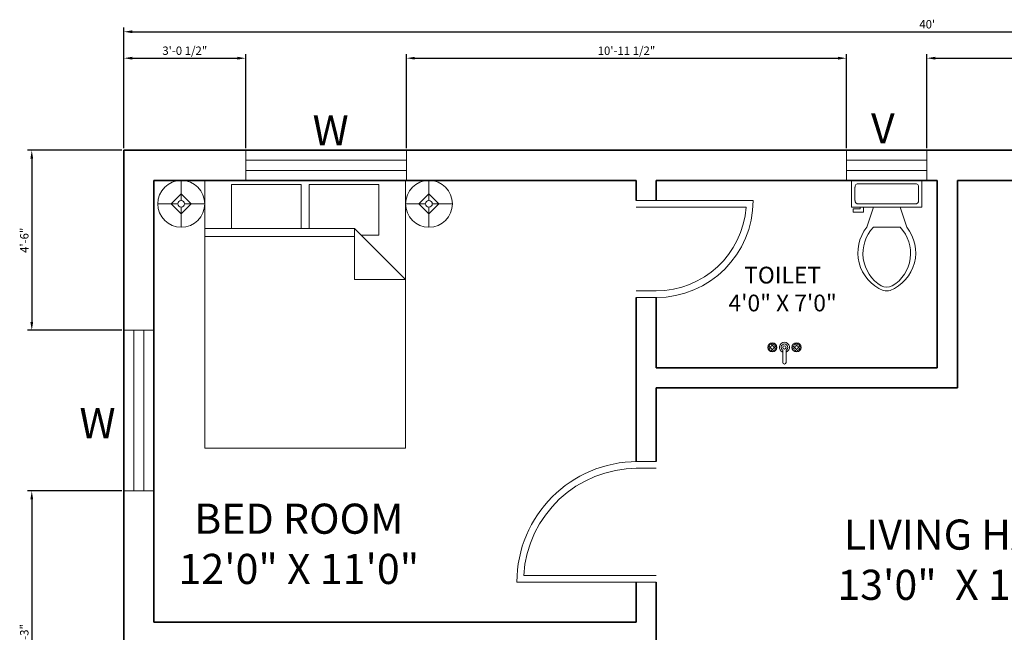
# Model space of a CAD drawing. Units: inches. Extents: x 1025 to 3479, y 1594 to 2212.
# Tile 8 of 9: x 2932 to 3226, y 1957 to 2140. Entities that reach past the tile are written whole.
import ezdxf

# ---------------------------------------------------------------- set-up
doc = ezdxf.new("R2010")
doc.units = ezdxf.units.IN
for name, color, linetype, lineweight in [('A-ANNO-DIMS', 1, 'Continuous', 18), ('A-ANNO-TEXT', 7, 'Continuous', 18), ('A-AREA-IDEN', 4, 'Continuous', 18), ('A-DOOR', 4, 'Continuous', 18), ('A-FLOR-FIXT', 9, 'Continuous', 18), ('A-FURN', 8, 'Continuous', 13), ('A-GLAZ', 3, 'Continuous', 18), ('A-WALL', 7, 'Continuous', 35)]:
    doc.layers.add(name, color=color, linetype=linetype, lineweight=lineweight)
doc.styles.get("Standard").update_dxf_attribs({"font": 'arial.ttf'})
doc.dimstyles.new('ISO-25', dxfattribs={"dimtxt": 2.5, "dimasz": 2.5, "dimexe": 1.25, "dimexo": 0.625, "dimtad": 1, "dimdec": 0, "dimlunit": 3, "dimtxsty": 'Standard', "dimcen": 2.5, "dimadec": 0, "dimazin": 0, "dimtfac": 1, "dimtdec": 0, "dimtmove": 0, "dimatfit": 3, "dimfxl": 1, "dimarcsym": 0})

# ---------------------------------------------------------------- blocks, each defined once
blk = doc.blocks.new('*D3')
at = {"layer": 'A-ANNO-DIMS', "color": 0, "lineweight": -2, "transparency": 16777216}
for p, q in [((2962.75, 2102.12), (2962.75, 2138.14)), ((2965.25, 2136.89), (3440.25, 2136.89)), ((3442.75, 2102.12), (3442.75, 2138.14))]:
    blk.add_line(p, q, dxfattribs=at)
at = {"layer": 'A-ANNO-DIMS', "color": 0, "transparency": 16777216}
for points in [[(2965.25, 2137.31), (2965.25, 2136.48), (2962.75, 2136.89)], [(3440.25, 2137.31), (3440.25, 2136.48), (3442.75, 2136.89)]]:
    blk.add_solid(points, dxfattribs=at)
at = {"layer": 'Defpoints', "color": 0, "transparency": 16777216}
for p in [(3442.75, 2136.89), (2962.75, 2101.49), (3442.75, 2101.49)]:
    blk.add_point(p, dxfattribs=at)
at = {"layer": 'A-ANNO-DIMS', "color": 0, "transparency": 16777216, "insert": (3202.75, 2138.8), "char_height": 2.5, "attachment_point": 5}
blk.add_mtext("40'", dxfattribs=at)
blk = doc.blocks.new('Bed - Queen')
for p, q in [((0, -80.00003), (0, 0)), ((0, 0), (59.99999, 0)), ((59.99999, 0), (59.99999, -80.00003)), ((7.99999, -1.2), (28.79998, -1.2)), ((7.99999, -14.4), (7.99999, -1.2)), ((28.79998, -1.2), (28.79998, -14.4)), ((31.19999, -1.2), (51.99999, -1.2)), ((31.19999, -14.4), (31.19999, -1.2)), ((51.99999, -1.2), (51.99999, -16.4)), ((0, -14.4), (44.8, -14.4)), ((59.99999, -29.6), (44.8, -14.4)), ((44.8, -14.4), (44.8, -29.6)), ((44.8, -16.8), (0, -16.8)), ((51.99999, -16.4), (46.79936, -16.4)), ((44.8, -29.6), (59.99999, -29.6)), ((59.99999, -80.00003), (0, -80.00003))]:
    blk.add_line(p, q)
blk = doc.blocks.new('Lamp - Table')
for p, q in [((0, 7), (0, 1)), ((0, 3), (-3, 0)), ((3, 0), (0, 3)), ((-1, 0), (-7, 0)), ((-3, 0), (0, -3)), ((0, -3), (3, 0)), ((1, 0), (7, 0)), ((0, -1), (0, -7))]:
    blk.add_line(p, q)
for radius in [7, 1]:
    blk.add_circle((0, 0), radius)
blk = doc.blocks.new('Toilet - top')
for p, q in [((9.5, -6), (9.5, -2)), ((-10, -8.5), (-8, -8.5)), ((-10, -9.5), (-10, -8.5)), ((-8, -8.5), (-8, -8)), ((-7, -8), (-7, -9.5)), ((-4, -8), (-6, -14)), ((4, -8), (6, -14)), ((-7, -9.5), (-10, -9.5)), ((4, -14), (-4, -14))]:
    blk.add_line(p, q)
blk.add_lwpolyline([(10.5, -8), (10.5, 0), (-10.5, 0), (-10.5, -8)], close=True)
for points in [[(-9.5, -2), (-9.5, -6)], [(8.5, -1), (-8.5, -1)], [(-8.5, -7), (8.5, -7)]]:
    blk.add_lwpolyline(points)
for centre, radius, start, end in [((-8.62, -1.88), 0.884, 81.8699, 188.1301), ((8.62, -1.88), 0.884, 351.8699, 98.1301), ((-8.62, -6.12), 0.884, 171.8699, 278.1301), ((8.62, -6.12), 0.884, 261.8699, 8.1301), ((3.52, -21.58), 12.17, 141.4691, 247.9714), ((4.2, -21.82), 11.33, 136.3677, 238.9468), ((-3.52, -21.58), 12.17, 292.0284, 38.5307), ((-4.2, -21.82), 11.33, 301.053, 43.6321), ((0, -27.88), 4, 245.7318, 294.2682), ((0, -29), 4, 254.8605, 285.1395)]:
    blk.add_arc(centre, radius, start, end)
blk = doc.blocks.new('Faucet - Bathroom top')
for p, q in [((-4.107, 0.125), (-4.375, 0.125)), ((-3.75, 0.4788), (-3.75, 0.75)), ((-3.5, 0.482), (-3.5, 0.75)), ((-3.1461, 0.125), (-2.875, 0.125)), ((3.143, 0.125), (2.875, 0.125)), ((3.5, 0.4788), (3.5, 0.75)), ((3.75, 0.482), (3.75, 0.75)), ((4.1039, 0.125), (4.375, 0.125)), ((-4.1039, -0.125), (-4.375, -0.125)), ((-3.75, -0.4821), (-3.75, -0.75)), ((-3.5, -0.4789), (-3.5, -0.75)), ((-3.143, -0.125), (-2.875, -0.125)), ((-0.5, -0.8639), (-0.5, -4.5)), ((0.5, -4.5), (0.5, -0.8631)), ((3.1461, -0.125), (2.875, -0.125)), ((3.5, -0.4821), (3.5, -0.75)), ((3.75, -0.4789), (3.75, -0.75)), ((4.107, -0.125), (4.375, -0.125))]:
    blk.add_line(p, q)
for centre, radius in [((-3.625, 0), 1.375), ((-4.625, 0), 0.2795), ((-3.625, 0), 0.5), ((-3.625, 1), 0.2795), ((-2.625, 0), 0.2795), ((0, 0), 0.5), ((3.625, 0), 1.375), ((2.625, 0), 0.2795), ((3.625, 0), 0.5), ((3.625, 1), 0.2795), ((4.625, 0), 0.2795), ((-3.625, -1), 0.2795), ((3.625, -1), 0.2795)]:
    blk.add_circle(centre, radius)
for centre, radius, start, end in [((-3.625, 0), 1, 105.2407, 164.2093), ((-3.625, 0), 1, 16.44125, 74.07887), ((0, 0), 1.5, 289.6514, 250.3603), ((0, 0), 1, 300.3431, 239.7554), ((3.625, 0), 1, 106.12, 164.0884), ((3.625, 0), 1, 16.23422, 73.90469), ((-3.625, 0), 1, 196.2342, 253.9047), ((-3.625, 0), 1, 286.12, 344.0884), ((3.625, 0), 1, 196.4413, 254.0789), ((3.625, 0), 1, 285.2407, 344.2093), ((0, -4.5), 0.5, 180, 0)]:
    blk.add_arc(centre, radius, start, end)
blk = doc.blocks.new('WIN-48IN')
for p, q in [((0, 48), (0, 0)), ((9, 48), (0, 48)), ((3, 48), (3, 0)), ((6, 0), (6, 48)), ((9, 0), (9, 48)), ((0, 0), (9, 0))]:
    blk.add_line(p, q)
blk = doc.blocks.new('VENT-24IN')
for p, q in [((24, 9), (0, 9)), ((0, 9), (0, 0)), ((24, 0), (24, 9)), ((24, 6), (0, 6)), ((0, 3), (24, 3)), ((0, 0), (24, 0))]:
    blk.add_line(p, q)
blk = doc.blocks.new('DOOR-SWING-29IN')
for p, q in [((0, 6), (0, 35)), ((2, 6), (2, 32.93)), ((0, 6), (0, 0)), ((2, 6), (2, 0)), ((27, 0), (27, 6)), ((29, 0), (29, 6))]:
    blk.add_line(p, q)
for radius, end in [(29, 90), (27, 85.752)]:
    blk.add_arc((0, 6), radius, 0, end)
blk = doc.blocks.new('*D61')
at = {"layer": 'A-ANNO-DIMS', "color": 0, "lineweight": -2, "transparency": 16777216}
for p, q in [((2962.75, 2102.12), (2962.75, 2130.24)), ((2999.18, 2102.12), (2999.18, 2130.24)), ((2965.25, 2128.99), (2996.68, 2128.99))]:
    blk.add_line(p, q, dxfattribs=at)
at = {"layer": 'A-ANNO-DIMS', "color": 0, "transparency": 16777216}
for points in [[(2965.25, 2129.41), (2965.25, 2128.58), (2962.75, 2128.99)], [(2996.68, 2129.41), (2996.68, 2128.58), (2999.18, 2128.99)]]:
    blk.add_solid(points, dxfattribs=at)
at = {"layer": 'Defpoints', "color": 0, "transparency": 16777216}
for p in [(2999.18, 2128.99), (2962.75, 2101.49), (2999.18, 2101.49)]:
    blk.add_point(p, dxfattribs=at)
at = {"layer": 'A-ANNO-DIMS', "color": 0, "transparency": 16777216, "insert": (2980.96, 2130.91), "char_height": 2.5, "attachment_point": 5}
blk.add_mtext('3\'-0 1/2"', dxfattribs=at)
blk = doc.blocks.new('*D62')
at = {"layer": 'A-ANNO-DIMS', "color": 0, "lineweight": -2, "transparency": 16777216}
for p, q in [((3047.18, 2102.12), (3047.18, 2130.24)), ((3178.62, 2102.12), (3178.62, 2130.24)), ((3049.68, 2128.99), (3176.12, 2128.99))]:
    blk.add_line(p, q, dxfattribs=at)
at = {"layer": 'A-ANNO-DIMS', "color": 0, "transparency": 16777216}
for points in [[(3049.68, 2129.41), (3049.68, 2128.58), (3047.18, 2128.99)], [(3176.12, 2129.41), (3176.12, 2128.58), (3178.62, 2128.99)]]:
    blk.add_solid(points, dxfattribs=at)
at = {"layer": 'Defpoints', "color": 0, "transparency": 16777216}
for p in [(3178.62, 2128.99), (3047.18, 2101.49), (3178.62, 2101.49)]:
    blk.add_point(p, dxfattribs=at)
at = {"layer": 'A-ANNO-DIMS', "color": 0, "transparency": 16777216, "insert": (3112.9, 2130.91), "char_height": 2.5, "attachment_point": 5}
blk.add_mtext('10\'-11 1/2"', dxfattribs=at)
blk = doc.blocks.new('*D63')
at = {"layer": 'A-ANNO-DIMS', "color": 0, "lineweight": -2, "transparency": 16777216}
for p, q in [((3202.62, 2102.12), (3202.62, 2130.24)), ((3303.38, 2102.12), (3303.38, 2130.24)), ((3205.12, 2128.99), (3300.88, 2128.99))]:
    blk.add_line(p, q, dxfattribs=at)
at = {"layer": 'A-ANNO-DIMS', "color": 0, "transparency": 16777216}
for points in [[(3205.12, 2129.41), (3205.12, 2128.58), (3202.62, 2128.99)], [(3300.88, 2129.41), (3300.88, 2128.58), (3303.38, 2128.99)]]:
    blk.add_solid(points, dxfattribs=at)
at = {"layer": 'Defpoints', "color": 0, "transparency": 16777216}
for p in [(3303.38, 2128.99), (3202.62, 2101.49), (3303.38, 2101.49)]:
    blk.add_point(p, dxfattribs=at)
at = {"layer": 'A-ANNO-DIMS', "color": 0, "transparency": 16777216, "insert": (3253, 2130.89), "char_height": 2.5, "attachment_point": 5}
blk.add_mtext('8\'-5"', dxfattribs=at)
blk = doc.blocks.new('*D65')
at = {"layer": 'A-ANNO-DIMS', "color": 0, "lineweight": -2, "transparency": 16777216}
for p, q in [((2962.12, 2101.49), (2934, 2101.49)), ((2935.25, 2098.99), (2935.25, 2050.21)), ((2962.12, 2047.71), (2934, 2047.71))]:
    blk.add_line(p, q, dxfattribs=at)
at = {"layer": 'A-ANNO-DIMS', "color": 0, "transparency": 16777216}
for points in [[(2934.83, 2098.99), (2935.66, 2098.99), (2935.25, 2101.49)], [(2934.83, 2050.21), (2935.66, 2050.21), (2935.25, 2047.71)]]:
    blk.add_solid(points, dxfattribs=at)
at = {"layer": 'Defpoints', "color": 0, "transparency": 16777216}
for p in [(2962.75, 2101.49), (2935.25, 2047.71), (2962.75, 2047.71)]:
    blk.add_point(p, dxfattribs=at)
at = {"layer": 'A-ANNO-DIMS', "color": 0, "transparency": 16777216, "insert": (2933.35, 2074.6), "char_height": 2.5, "attachment_point": 5, "rotation": 90}
blk.add_mtext('4\'-6"', dxfattribs=at)
blk = doc.blocks.new('*D66')
at = {"layer": 'A-ANNO-DIMS', "color": 0, "lineweight": -2, "transparency": 16777216}
for p, q in [((2962.12, 1999.71), (2934, 1999.71)), ((2935.25, 1997.21), (2935.25, 1915.15)), ((2962.12, 1912.65), (2934, 1912.65))]:
    blk.add_line(p, q, dxfattribs=at)
at = {"layer": 'A-ANNO-DIMS', "color": 0, "transparency": 16777216}
for points in [[(2934.83, 1997.21), (2935.66, 1997.21), (2935.25, 1999.71)], [(2934.83, 1915.15), (2935.66, 1915.15), (2935.25, 1912.65)]]:
    blk.add_solid(points, dxfattribs=at)
at = {"layer": 'Defpoints', "color": 0, "transparency": 16777216}
for p in [(2962.75, 1999.71), (2935.25, 1912.65), (2962.75, 1912.65)]:
    blk.add_point(p, dxfattribs=at)
at = {"layer": 'A-ANNO-DIMS', "color": 0, "transparency": 16777216, "insert": (2933.34, 1956.18), "char_height": 2.5, "attachment_point": 5, "rotation": 90}
blk.add_mtext('7\'-3"', dxfattribs=at)

msp = doc.modelspace()

# ---------------------------------------------------------------- linework, layer by layer
at = {"layer": 'A-DOOR'}
for p, q in [((3150.68, 2084.49), (3150.75, 2084.49)), ((3115.75, 2057.49), (3121.75, 2057.49)), ((3121.75, 2008.49), (3115.75, 2008.49)), ((3121.75, 2006.49), (3115.75, 2006.49)), ((3080.22, 1974.49), (3080.17, 1974.49)), ((3115.75, 1974.49), (3082.23, 1974.49)), ((3115.75, 1974.49), (3121.75, 1974.49)), ((3115.75, 1972.49), (3080.17, 1972.49)), ((3115.75, 1972.49), (3121.75, 1972.49))]:
    msp.add_line(p, q, dxfattribs=at)
for radius, end in [(36, 180), (34, 176.6277)]:
    msp.add_arc((3116.17, 1972.49), radius, 90, end, dxfattribs=at)
at = {"layer": 'A-WALL'}
for p, q in [((2962.75, 2101.49), (3442.75, 2101.49)), ((2962.75, 1741.49), (2962.75, 2101.49)), ((2971.75, 2092.49), (3115.75, 2092.49)), ((2971.75, 1960.49), (2971.75, 2092.49)), ((3115.75, 2092.49), (3115.75, 2086.49)), ((3115.75, 2086.49), (3115.75, 2092.49)), ((3121.75, 2092.49), (3205.75, 2092.49)), ((3121.75, 2086.49), (3121.75, 2092.49)), ((3205.75, 2036.49), (3205.75, 2092.49)), ((3211.75, 2036.49), (3211.75, 2092.49)), ((3211.75, 2092.49), (3241.75, 2092.49)), ((3115.75, 2008.49), (3115.75, 2057.49)), ((3121.75, 2036.49), (3121.75, 2057.49)), ((3121.75, 2036.49), (3205.75, 2036.49)), ((3211.75, 2036.49), (3211.75, 2030.49)), ((3121.75, 2030.49), (3211.75, 2030.49)), ((3121.75, 2008.49), (3121.75, 2030.49)), ((3115.75, 1960.49), (3115.75, 1972.49)), ((3115.75, 1960.49), (3115.75, 1972.49)), ((3121.75, 1942.49), (3121.75, 1972.49)), ((2971.75, 1960.49), (3115.75, 1960.49))]:
    msp.add_line(p, q, dxfattribs=at)

# ---------------------------------------------------------------- block references
at = {"layer": 'A-DOOR', "rotation": 270.0000000000028}
msp.add_blockref('DOOR-SWING-29IN', (3115.75, 2086.49), dxfattribs=at)
at = {"layer": 'A-FLOR-FIXT'}
for name, p in [('Toilet - top', (3190.67, 2092.49)), ('Faucet - Bathroom top', (3160.09, 2042.62))]:
    msp.add_blockref(name, p, dxfattribs=at)
at = {"layer": 'A-FURN'}
for name, p in [('Lamp - Table', (2979.9, 2085.49)), ('Bed - Queen', (2986.9, 2092.49)), ('Lamp - Table', (3053.9, 2085.49))]:
    msp.add_blockref(name, p, dxfattribs=at)
at = {"layer": 'A-GLAZ', "rotation": 270.0000000000021}
msp.add_blockref('WIN-48IN', (2999.18, 2101.49), dxfattribs=at)
at = {"layer": 'A-GLAZ'}
for name, p in [('VENT-24IN', (3178.62, 2092.49)), ('WIN-48IN', (2962.75, 1999.71))]:
    msp.add_blockref(name, p, dxfattribs=at)

# ---------------------------------------------------------------- texts
at = {"layer": 'A-ANNO-TEXT', "char_height": 9, "attachment_point": 1}
for s, width, insert in [('\\pxqc;W', 15.8719, (3016.6, 2111.93)), ('\\pxqc;{V}', 7.8272, (3185.58, 2112.55)), ('\\pxqc;W', 15.8719, (2946.95, 2024.48))]:
    msp.add_mtext_dynamic_manual_height_columns(s, width=width, gutter_width=12.5, heights=[0], dxfattribs=dict(at, insert=insert))
at = {"layer": 'A-AREA-IDEN', "attachment_point": 1}
for s, width, insert, char_height in [('\\pxqc;TOILET \\P4\'0" X 7\'0" ', 51.1118, (3133.99, 2066.7), 5), ('\\pxqc;BED ROOM \\P12\'0" X 11\'0"', 93.2353, (2968.42, 1995.93), 9), ('\\pxqc;LIVING HALL \\P13\'0"  X 17\'0"', 93.2353, (3166.61, 1991.18), 9)]:
    msp.add_mtext_dynamic_manual_height_columns(s, width=width, gutter_width=12.5, heights=[0], dxfattribs=dict(at, insert=insert, char_height=char_height))

# ---------------------------------------------------------------- dimensions: what is measured, and where the dimension line sits
at = {"layer": 'A-ANNO-DIMS'}
for base, p1, p2, override, picture, middle in [((3442.75, 2136.89), (2962.75, 2101.49), (3442.75, 2101.49), {"dimclrd": 0, "dimclre": 0, "dimclrt": 0}, '*D3', (3202.75, 2138.8)), ((2999.18, 2128.99), (2962.75, 2101.49), (2999.18, 2101.49), {"dimdec": 1, "dimlfac": 1, "dimrnd": 0, "dimzin": 1, "dimdsep": 46, "dimlunit": 4, "dimfrac": 2}, '*D61', (2980.96, 2130.91)), ((3178.62, 2128.99), (3047.18, 2101.49), (3178.62, 2101.49), {"dimdec": 1, "dimlfac": 1, "dimrnd": 0, "dimzin": 1, "dimdsep": 46, "dimlunit": 4, "dimfrac": 2}, '*D62', (3112.9, 2130.91)), ((3303.38, 2128.99), (3202.62, 2101.49), (3303.38, 2101.49), {"dimdec": 1, "dimlfac": 1, "dimrnd": 0, "dimzin": 1, "dimdsep": 46, "dimlunit": 4, "dimfrac": 2}, '*D63', (3253, 2130.89))]:
    dim = msp.add_linear_dim(base=base, p1=p1, p2=p2, dimstyle='ISO-25', override=override, dxfattribs=at)
    dim.commit()
    dim.dimension.update_dxf_attribs({"geometry": picture, "text_midpoint": middle})
for base, p1, p2, picture, middle in [((2935.25, 2047.71), (2962.75, 2101.49), (2962.75, 2047.71), '*D65', (2933.35, 2074.6)), ((2935.25, 1912.65), (2962.75, 1999.71), (2962.75, 1912.65), '*D66', (2933.34, 1956.18))]:
    dim = msp.add_linear_dim(base=base, p1=p1, p2=p2, angle=90, dimstyle='ISO-25', override={"dimdec": 1, "dimlfac": 1, "dimrnd": 0, "dimzin": 1, "dimdsep": 46, "dimlunit": 4, "dimfrac": 2}, dxfattribs=at)
    dim.commit()
    dim.dimension.update_dxf_attribs({"geometry": picture, "text_midpoint": middle})

doc.saveas('drawing.dxf')
